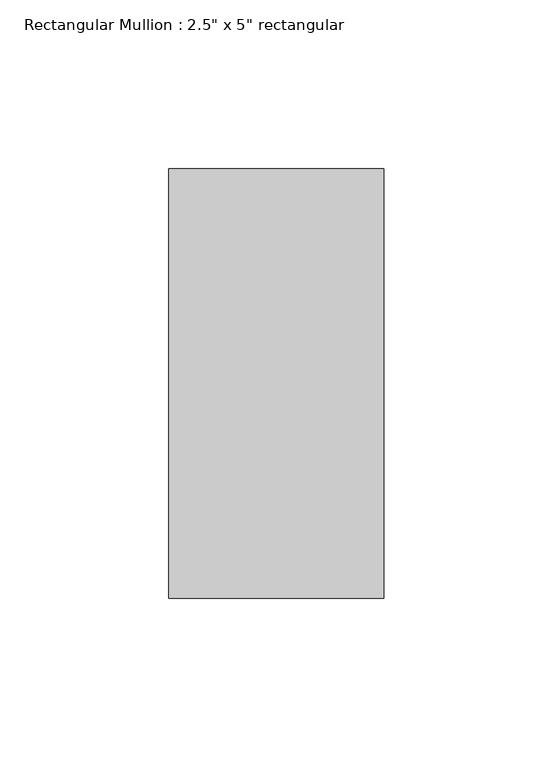
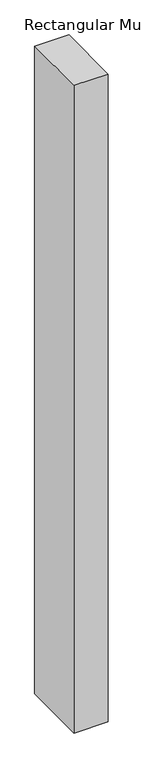
"""IFC4 building model written with IfcOpenShell, lengths in millimetres: member geometry."""

from ifc_helpers import new_model, si_unit, frame, origin, place, context, project, spatial, polyline, outline, extrude, source, transform, mapped, element, save


def member_f066cb84(model_context):
    return source(origin(), model_context, "Body", "SweptSolid", [
        extrude(outline(polyline([(31.75, 63.5), (31.75, -63.5), (-31.75, -63.5), (-31.75, 63.5), (31.75, 63.5)])), frame((0.0, 0.0, -1274.1056645), z_axis=(0.0, 0.0, 1.0), x_axis=(1.0, 0.0, 0.0)), (0.0, 0.0, 1.0), 1274.1056645),
    ])


if __name__ == "__main__":
    model = new_model("IFC4")
    model_context = context("Model", 3, world=origin())
    ifc_project = project(units=[si_unit("LENGTHUNIT", "METRE", prefix="MILLI")], contexts=[model_context])
    site = spatial("IfcSite", under=ifc_project)
    building = spatial("IfcBuilding", under=site)
    placement = place(None, origin())
    member_shape = member_f066cb84(model_context)
    element("IfcMember", 1, ObjectType="Rectangular Mullion : 2.5\" x 5\" rectangular", at=placement, inside=building, context=model_context, shape_type="MappedRepresentation", body=[
        mapped(member_shape, transform((0.0, 0.0, 0.0), x_axis=(1.0, 0.0, 0.0), y_axis=(0.0, 1.0, 0.0), z_axis=(0.0, 0.0, 1.0))),
    ])
    save(model, "model.ifc")

# Revit data of these elements
# Type "Rectangular Mullion : 2.5\" x 5\" rectangular"
#   built-in parameter 1007304 = 0.416667 (stored number, unit not read)
#   built-in parameter 1007301 = 0.104167 (stored number, unit not read)
#   built-in parameter 1007300 = 0.104167 (stored number, unit not read)
